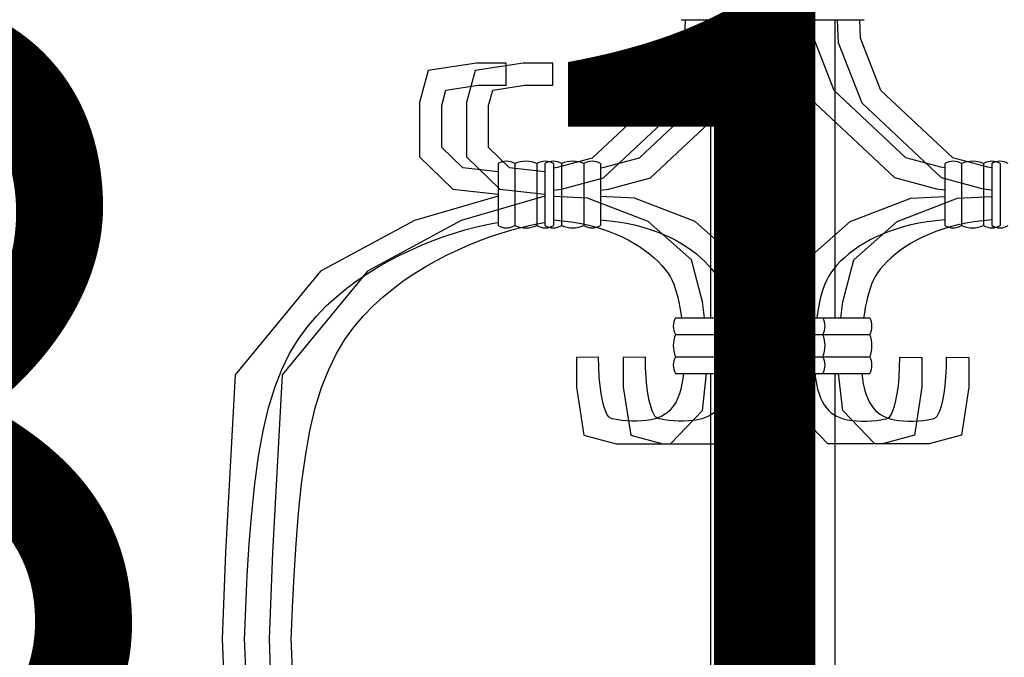
# Model space of a CAD drawing. Units: inches. Extents: x 2278 to 7495, y -71 to 1198.
# Tile 32 of 44: x 5127.04 to 5134.27, y 141.192 to 145.876. Entities that reach past the tile are written whole.
import ezdxf

# ---------------------------------------------------------------- set-up
doc = ezdxf.new("R2010")
doc.units = ezdxf.units.IN
doc.header["$MEASUREMENT"] = 0
doc.layers.add('A-ANNO-DIMS', color=2, linetype='Continuous', lineweight=18)
doc.layers.add('A-ELEV', color=7, linetype='Continuous', lineweight=25)
doc.styles.get("Standard").update_dxf_attribs({"font": 'arial.ttf'})
doc.dimstyles.get("Standard").update_dxf_attribs({"dimtxt": 6, "dimasz": 3, "dimexe": 0.18, "dimexo": 0.0625, "dimgap": 0.09, "dimtad": 0, "dimtih": 1, "dimtoh": 1, "dimdec": 0, "dimzin": 0, "dimdsep": 46, "dimlunit": 3, "dimtxsty": 'Standard', "dimblk": 'ARCHTICK', "dimcen": 0.09, "dimadec": 0, "dimazin": 0, "dimtfac": 1, "dimtdec": 0, "dimtofl": 0, "dimtmove": 0, "dimatfit": 3, "dimfxl": 1, "dimtolj": 1, "dimtzin": 0, "dimarcsym": 0})

# ---------------------------------------------------------------- blocks, each defined once
blk = doc.blocks.new('_ArchTick')
at = {"color": 0, "linetype": 'ByBlock', "const_width": 0.15}
blk.add_lwpolyline([(-0.5, -0.5), (0.5, 0.5)], dxfattribs=at)
blk = doc.blocks.new('*D59')
at = {"layer": 'A-ANNO-DIMS', "color": 0, "lineweight": -2, "transparency": 16777216}
for p, q in [((5096.5894, 159.1826), (5101.5644, 159.1826)), ((5101.3844, 159.1826), (5101.3844, 146.185)), ((5101.3844, 126.7988), (5101.3844, 139.7963)), ((5096.5894, 126.7988), (5101.5644, 126.7988))]:
    blk.add_line(p, q, dxfattribs=at)
at = {"layer": 'Defpoints', "color": 0, "transparency": 16777216}
for p in [(5096.5269, 159.1826), (5101.3844, 159.1826), (5096.5269, 126.7988)]:
    blk.add_point(p, dxfattribs=at)
at = {"layer": 'A-ANNO-DIMS', "color": 0, "lineweight": -2, "transparency": 16777216, "xscale": 3, "yscale": 3, "zscale": 3}
for p, rotation in [((5101.3844, 159.1826), 90), ((5101.3844, 126.7988), 270)]:
    blk.add_blockref('_ArchTick', p, dxfattribs=dict(at, rotation=rotation))
at = {"layer": 'A-ANNO-DIMS', "color": 0, "transparency": 16777216, "insert": (5101.3844, 142.9907), "char_height": 6, "attachment_point": 5}
blk.add_mtext('\\A1;ORNATE BALUSTER 2\'-8 1/2" TYP.', dxfattribs=at)
blk = doc.blocks.new('*D123')
at = {"layer": 'A-ANNO-DIMS', "color": 0, "lineweight": -2, "transparency": 16777216}
for p, q in [((4736.95, 340.1567), (4736.95, -23.4272)), ((5145.6762, -1.8097), (5145.6762, -23.4272)), ((4736.95, -23.2472), (4923.9291, -23.2472)), ((5145.6762, -23.2472), (4958.6971, -23.2472))]:
    blk.add_line(p, q, dxfattribs=at)
at = {"layer": 'Defpoints', "color": 0, "transparency": 16777216}
for p in [(4736.95, 340.2192), (5145.6762, -1.7472), (5145.6762, -23.2472)]:
    blk.add_point(p, dxfattribs=at)
at = {"layer": 'A-ANNO-DIMS', "color": 0, "lineweight": -2, "transparency": 16777216, "xscale": 3, "yscale": 3, "zscale": 3, "rotation": 180}
blk.add_blockref('_ArchTick', (4736.95, -23.2472), dxfattribs=at)
at = {"layer": 'A-ANNO-DIMS', "color": 0, "lineweight": -2, "transparency": 16777216, "xscale": 3, "yscale": 3, "zscale": 3}
blk.add_blockref('_ArchTick', (5145.6762, -23.2472), dxfattribs=at)
at = {"layer": 'A-ANNO-DIMS', "color": 0, "transparency": 16777216, "insert": (4941.3131, -23.2472), "char_height": 6, "attachment_point": 5}
blk.add_mtext('\\A1;34\'-0 1/2"', dxfattribs=at)
blk = doc.blocks.new('*D131')
at = {"layer": 'A-ANNO-DIMS', "color": 0, "lineweight": -2, "transparency": 16777216}
for p, q in [((5096.1762, 99.3153), (5096.1762, 361.8992)), ((5145.6762, 118.3153), (5145.6762, 361.8992)), ((5096.1762, 361.7192), (5105.7503, 361.7192)), ((5145.6762, 361.7192), (5136.1022, 361.7192))]:
    blk.add_line(p, q, dxfattribs=at)
at = {"layer": 'Defpoints', "color": 0, "transparency": 16777216}
for p in [(5145.6762, 361.7192), (5145.6762, 118.2528), (5096.1762, 99.2528)]:
    blk.add_point(p, dxfattribs=at)
at = {"layer": 'A-ANNO-DIMS', "color": 0, "lineweight": -2, "transparency": 16777216, "xscale": 3, "yscale": 3, "zscale": 3, "rotation": 180}
blk.add_blockref('_ArchTick', (5096.1762, 361.7192), dxfattribs=at)
at = {"layer": 'A-ANNO-DIMS', "color": 0, "lineweight": -2, "transparency": 16777216, "xscale": 3, "yscale": 3, "zscale": 3}
blk.add_blockref('_ArchTick', (5145.6762, 361.7192), dxfattribs=at)
at = {"layer": 'A-ANNO-DIMS', "color": 0, "transparency": 16777216, "insert": (5120.9262, 361.7192), "char_height": 6, "attachment_point": 5}
blk.add_mtext('\\A1;4\'-1 1/2"', dxfattribs=at)
blk = doc.blocks.new('*D139')
at = {"layer": 'A-ANNO-DIMS', "color": 0, "lineweight": -2, "transparency": 16777216}
for p, q in [((5092.2387, 160.2528), (5167.7538, 160.2528)), ((5167.5738, 160.2528), (5167.5738, 142.4083)), ((5167.5738, 118.2528), (5167.5738, 136.0973)), ((5145.7387, 118.2528), (5167.7538, 118.2528))]:
    blk.add_line(p, q, dxfattribs=at)
at = {"layer": 'Defpoints', "color": 0, "transparency": 16777216}
for p in [(5092.1762, 160.2528), (5167.5738, 160.2528), (5145.6762, 118.2528)]:
    blk.add_point(p, dxfattribs=at)
at = {"layer": 'A-ANNO-DIMS', "color": 0, "lineweight": -2, "transparency": 16777216, "xscale": 3, "yscale": 3, "zscale": 3}
for p, rotation in [((5167.5738, 160.2528), 90), ((5167.5738, 118.2528), 270)]:
    blk.add_blockref('_ArchTick', p, dxfattribs=dict(at, rotation=rotation))
at = {"layer": 'A-ANNO-DIMS', "color": 0, "transparency": 16777216, "insert": (5167.5738, 139.2528), "char_height": 6, "attachment_point": 5}
blk.add_mtext('\\A1;3\'-6"', dxfattribs=at)

msp = doc.modelspace()

# ---------------------------------------------------------------- linework, layer by layer
at = {"layer": 'A-ELEV'}
for p, q in [((5131.8965, 145.8765), (5132.8966, 145.8765)), ((5131.9226, 145.7411), (5131.9286, 145.8765)), ((5132.0842, 145.7072), (5132.0917, 145.8765)), ((5132.1114, 145.8765), (5132.1114, 143.6856)), ((5132.2404, 145.8765), (5133.2405, 145.8765)), ((5132.2665, 145.7411), (5132.2725, 145.8765)), ((5132.4281, 145.7072), (5132.4356, 145.8765)), ((5132.4553, 145.8765), (5132.4553, 143.6856)), ((5132.6817, 145.8765), (5132.6817, 143.6856)), ((5132.7089, 145.7072), (5132.7015, 145.8765)), ((5132.8705, 145.7411), (5132.8646, 145.8765)), ((5133.0256, 145.8765), (5133.0256, 143.6856)), ((5133.0528, 145.7072), (5133.0454, 145.8765)), ((5133.2144, 145.7411), (5133.2085, 145.8765)), ((5131.7733, 145.3557), (5131.9226, 145.7411)), ((5131.9118, 145.2623), (5132.0842, 145.7072)), ((5132.1172, 145.3557), (5132.2665, 145.7411)), ((5132.2557, 145.2623), (5132.4281, 145.7072)), ((5132.8813, 145.2623), (5132.7089, 145.7072)), ((5133.0199, 145.3557), (5132.8705, 145.7411)), ((5133.2252, 145.2623), (5133.0528, 145.7072)), ((5133.3638, 145.3557), (5133.2144, 145.7411)), ((5130.393, 145.5581), (5130.0391, 145.5036)), ((5130.7369, 145.5581), (5130.383, 145.5036)), ((5130.6107, 145.5581), (5130.393, 145.5581)), ((5130.6107, 145.3952), (5130.6107, 145.5581)), ((5130.9546, 145.5581), (5130.7369, 145.5581)), ((5130.9546, 145.3952), (5130.9546, 145.5581)), ((5130.0391, 145.5036), (5129.9756, 145.2675)), ((5130.383, 145.5036), (5130.3195, 145.2675)), ((5130.1386, 145.246), (5130.1689, 145.3587)), ((5130.1689, 145.3587), (5130.4054, 145.3952)), ((5130.4054, 145.3952), (5130.6107, 145.3952)), ((5130.4825, 145.246), (5130.5128, 145.3587)), ((5130.5128, 145.3587), (5130.7493, 145.3952)), ((5130.7493, 145.3952), (5130.9546, 145.3952)), ((5131.2459, 144.8607), (5131.7733, 145.3557)), ((5131.5898, 144.8607), (5132.1172, 145.3557)), ((5133.5472, 144.8607), (5133.0199, 145.3557)), ((5133.8911, 144.8607), (5133.3638, 145.3557)), ((5129.9756, 145.2675), (5129.9756, 144.868)), ((5130.3195, 145.2675), (5130.3195, 144.868)), ((5131.3274, 144.7137), (5131.9118, 145.2623)), ((5131.6713, 144.7137), (5132.2557, 145.2623)), ((5133.4657, 144.7137), (5132.8813, 145.2623)), ((5133.8096, 144.7137), (5133.2252, 145.2623)), ((5130.1386, 144.9373), (5130.1386, 145.246)), ((5130.4825, 144.9373), (5130.4825, 145.246)), ((5130.2936, 144.7879), (5130.1386, 144.9373)), ((5130.6375, 144.7879), (5130.4825, 144.9373)), ((5129.9756, 144.868), (5130.2206, 144.632)), ((5130.3195, 144.868), (5130.5645, 144.632)), ((5130.5528, 144.8198), (5130.5528, 144.3639)), ((5130.675, 144.8198), (5130.675, 144.3639)), ((5130.838, 144.8198), (5130.838, 144.3639)), ((5130.8967, 144.8198), (5130.8967, 144.3639)), ((5130.9602, 144.8198), (5130.9602, 144.3639)), ((5130.9883, 144.7924), (5131.2459, 144.8607)), ((5131.0189, 144.8198), (5131.0189, 144.3639)), ((5131.1819, 144.8198), (5131.1819, 144.3639)), ((5131.3041, 144.8198), (5131.3041, 144.3639)), ((5131.3322, 144.7924), (5131.5898, 144.8607)), ((5133.8048, 144.7924), (5133.5472, 144.8607)), ((5133.833, 144.8198), (5133.833, 144.3639)), ((5134.1487, 144.7924), (5133.8911, 144.8607)), ((5133.9552, 144.8198), (5133.9552, 144.3639)), ((5134.1181, 144.8198), (5134.1181, 144.3639)), ((5134.1769, 144.8198), (5134.1769, 144.3639)), ((5134.2403, 144.8198), (5134.2403, 144.3639)), ((5130.5528, 144.7597), (5130.2936, 144.7879)), ((5130.8967, 144.7597), (5130.6375, 144.7879)), ((5130.9602, 144.7891), (5130.9883, 144.7924)), ((5131.3041, 144.7891), (5131.3322, 144.7924)), ((5133.833, 144.7891), (5133.8048, 144.7924)), ((5134.1769, 144.7891), (5134.1487, 144.7924)), ((5131.019, 144.632), (5131.3274, 144.7137)), ((5131.3629, 144.632), (5131.6713, 144.7137)), ((5133.7742, 144.632), (5133.4657, 144.7137)), ((5134.1181, 144.632), (5133.8096, 144.7137)), ((5130.2206, 144.632), (5130.5528, 144.5958)), ((5130.5645, 144.632), (5130.8967, 144.5958)), ((5130.9602, 144.625), (5131.019, 144.632)), ((5131.3041, 144.625), (5131.3629, 144.632)), ((5133.833, 144.625), (5133.7742, 144.632)), ((5134.1769, 144.625), (5134.1181, 144.632)), ((5130.5528, 144.581), (5129.9387, 144.402)), ((5130.8967, 144.581), (5130.2826, 144.402)), ((5131.2098, 144.5653), (5130.9602, 144.5763)), ((5131.6547, 144.3929), (5131.2098, 144.5653)), ((5131.5537, 144.5653), (5131.3041, 144.5763)), ((5131.9986, 144.3929), (5131.5537, 144.5653)), ((5133.1384, 144.3929), (5133.5833, 144.5653)), ((5133.4823, 144.3929), (5133.9272, 144.5653)), ((5133.5833, 144.5653), (5133.833, 144.5763)), ((5133.9272, 144.5653), (5134.1769, 144.5763)), ((5129.9387, 144.402), (5129.2486, 144.03)), ((5130.2826, 144.402), (5129.5925, 144.03)), ((5130.5338, 144.3836), (5130.5528, 144.3865)), ((5130.8777, 144.3836), (5130.8967, 144.3865)), ((5130.9602, 144.405), (5131.0258, 144.3993)), ((5131.0258, 144.3993), (5131.0896, 144.3912)), ((5131.0896, 144.3912), (5131.1509, 144.3809)), ((5131.3041, 144.405), (5131.3697, 144.3993)), ((5131.3697, 144.3993), (5131.4335, 144.3912)), ((5131.4335, 144.3912), (5131.4948, 144.3809)), ((5131.9725, 144.1117), (5131.6547, 144.3929)), ((5132.3164, 144.1117), (5131.9986, 144.3929)), ((5132.8207, 144.1117), (5133.1384, 144.3929)), ((5133.1646, 144.1117), (5133.4823, 144.3929)), ((5133.7035, 144.3912), (5133.6422, 144.3809)), ((5133.7673, 144.3993), (5133.7035, 144.3912)), ((5133.833, 144.405), (5133.7673, 144.3993)), ((5134.0474, 144.3912), (5133.9861, 144.3809)), ((5134.1112, 144.3993), (5134.0474, 144.3912)), ((5134.1769, 144.405), (5134.1112, 144.3993)), ((5130.2316, 144.3089), (5130.3086, 144.3322)), ((5130.3086, 144.3322), (5130.3846, 144.3524)), ((5130.3846, 144.3524), (5130.4597, 144.3696)), ((5130.4597, 144.3696), (5130.5338, 144.3836)), ((5130.5755, 144.3089), (5130.6525, 144.3322)), ((5130.6525, 144.3322), (5130.7285, 144.3524)), ((5130.7285, 144.3524), (5130.8036, 144.3696)), ((5130.8036, 144.3696), (5130.8777, 144.3836)), ((5131.1509, 144.3809), (5131.2094, 144.3687)), ((5131.2094, 144.3687), (5131.2652, 144.3546)), ((5131.2652, 144.3546), (5131.3184, 144.3387)), ((5131.3184, 144.3387), (5131.3691, 144.3211)), ((5131.3691, 144.3211), (5131.4175, 144.3018)), ((5131.4948, 144.3809), (5131.5534, 144.3687)), ((5131.5534, 144.3687), (5131.6091, 144.3546)), ((5131.6091, 144.3546), (5131.6623, 144.3387)), ((5131.6623, 144.3387), (5131.713, 144.3211)), ((5131.713, 144.3211), (5131.7614, 144.3018)), ((5133.424, 144.3211), (5133.3756, 144.3018)), ((5133.4747, 144.3387), (5133.424, 144.3211)), ((5133.5279, 144.3546), (5133.4747, 144.3387)), ((5133.5837, 144.3687), (5133.5279, 144.3546)), ((5133.6422, 144.3809), (5133.5837, 144.3687)), ((5133.7679, 144.3211), (5133.7195, 144.3018)), ((5133.8186, 144.3387), (5133.7679, 144.3211)), ((5133.8718, 144.3546), (5133.8186, 144.3387)), ((5133.9276, 144.3687), (5133.8718, 144.3546)), ((5133.9861, 144.3809), (5133.9276, 144.3687)), ((5129.9956, 144.2214), (5130.0751, 144.2535)), ((5130.0751, 144.2535), (5130.1538, 144.2827)), ((5130.1538, 144.2827), (5130.2316, 144.3089)), ((5130.3395, 144.2214), (5130.419, 144.2535)), ((5130.419, 144.2535), (5130.4977, 144.2827)), ((5130.4977, 144.2827), (5130.5755, 144.3089)), ((5131.4175, 144.3018), (5131.4637, 144.281)), ((5131.4637, 144.281), (5131.5079, 144.2586)), ((5131.5079, 144.2586), (5131.5502, 144.2347)), ((5131.7614, 144.3018), (5131.8076, 144.281)), ((5131.8076, 144.281), (5131.8518, 144.2586)), ((5131.8518, 144.2586), (5131.8941, 144.2347)), ((5133.2852, 144.2586), (5133.2429, 144.2347)), ((5133.3294, 144.281), (5133.2852, 144.2586)), ((5133.3756, 144.3018), (5133.3294, 144.281)), ((5133.6291, 144.2586), (5133.5868, 144.2347)), ((5133.6733, 144.281), (5133.6291, 144.2586)), ((5133.7195, 144.3018), (5133.6733, 144.281)), ((5129.8357, 144.149), (5129.9156, 144.1867)), ((5129.9156, 144.1867), (5129.9956, 144.2214)), ((5130.1796, 144.149), (5130.2595, 144.1867)), ((5130.2595, 144.1867), (5130.3395, 144.2214)), ((5131.5502, 144.2347), (5131.5906, 144.2094)), ((5131.5906, 144.2094), (5131.6288, 144.183)), ((5131.6288, 144.183), (5131.6645, 144.1557)), ((5131.8941, 144.2347), (5131.9345, 144.2094)), ((5131.9345, 144.2094), (5131.9727, 144.183)), ((5131.9727, 144.183), (5132.0084, 144.1557)), ((5133.1644, 144.183), (5133.1286, 144.1557)), ((5133.2026, 144.2094), (5133.1644, 144.183)), ((5133.2429, 144.2347), (5133.2026, 144.2094)), ((5133.5083, 144.183), (5133.4725, 144.1557)), ((5133.5465, 144.2094), (5133.5083, 144.183)), ((5133.5868, 144.2347), (5133.5465, 144.2094)), ((5129.6768, 144.0636), (5129.7561, 144.1081)), ((5129.7561, 144.1081), (5129.8357, 144.149)), ((5130.0207, 144.0636), (5130.1, 144.1081)), ((5130.1, 144.1081), (5130.1796, 144.149)), ((5131.6645, 144.1557), (5131.6975, 144.1278)), ((5131.6975, 144.1278), (5131.7276, 144.0995)), ((5131.7276, 144.0995), (5131.7545, 144.0712)), ((5132.0542, 143.8032), (5131.9725, 144.1117)), ((5132.0084, 144.1557), (5132.0414, 144.1278)), ((5132.0414, 144.1278), (5132.0715, 144.0995)), ((5132.0715, 144.0995), (5132.0984, 144.0712)), ((5132.3981, 143.8032), (5132.3164, 144.1117)), ((5132.7389, 143.8032), (5132.8207, 144.1117)), ((5133.0655, 144.0995), (5133.0386, 144.0712)), ((5133.0956, 144.1278), (5133.0655, 144.0995)), ((5133.0828, 143.8032), (5133.1646, 144.1117)), ((5133.1286, 144.1557), (5133.0956, 144.1278)), ((5133.4094, 144.0995), (5133.3825, 144.0712)), ((5133.4395, 144.1278), (5133.4094, 144.0995)), ((5133.4725, 144.1557), (5133.4395, 144.1278)), ((5129.2486, 144.03), (5128.6221, 143.2679)), ((5129.5925, 144.03), (5128.966, 143.2679)), ((5129.598, 144.0151), (5129.6768, 144.0636)), ((5129.942, 144.0151), (5130.0207, 144.0636)), ((5131.7545, 144.0712), (5131.7781, 144.0431)), ((5131.7781, 144.0431), (5131.7981, 144.0157)), ((5132.0984, 144.0712), (5132.122, 144.0431)), ((5132.122, 144.0431), (5132.142, 144.0157)), ((5133.0151, 144.0431), (5132.995, 144.0157)), ((5133.0386, 144.0712), (5133.0151, 144.0431)), ((5133.359, 144.0431), (5133.3389, 144.0157)), ((5133.3825, 144.0712), (5133.359, 144.0431)), ((5129.4423, 143.9045), (5129.5199, 143.9622)), ((5129.5199, 143.9622), (5129.598, 144.0151)), ((5129.7862, 143.9045), (5129.8638, 143.9622)), ((5129.8638, 143.9622), (5129.942, 144.0151)), ((5131.7981, 144.0157), (5131.815, 143.9886)), ((5131.815, 143.9886), (5131.8296, 143.9612)), ((5131.8296, 143.9612), (5131.8422, 143.9327)), ((5132.142, 144.0157), (5132.159, 143.9886)), ((5132.159, 143.9886), (5132.1735, 143.9612)), ((5132.1735, 143.9612), (5132.1861, 143.9327)), ((5132.9635, 143.9612), (5132.9509, 143.9327)), ((5132.9781, 143.9886), (5132.9635, 143.9612)), ((5132.995, 144.0157), (5132.9781, 143.9886)), ((5133.3074, 143.9612), (5133.2948, 143.9327)), ((5133.322, 143.9886), (5133.3074, 143.9612)), ((5133.3389, 144.0157), (5133.322, 143.9886)), ((5129.3657, 143.8416), (5129.4423, 143.9045)), ((5129.7096, 143.8416), (5129.7862, 143.9045)), ((5131.8422, 143.9327), (5131.8534, 143.9027)), ((5131.8534, 143.9027), (5131.8633, 143.8709)), ((5132.1861, 143.9327), (5132.1973, 143.9027)), ((5132.1973, 143.9027), (5132.2072, 143.8709)), ((5132.9397, 143.9027), (5132.9298, 143.8709)), ((5132.9509, 143.9327), (5132.9397, 143.9027)), ((5133.2836, 143.9027), (5133.2737, 143.8709)), ((5133.2948, 143.9327), (5133.2836, 143.9027)), ((5129.2908, 143.7735), (5129.3657, 143.8416)), ((5129.6347, 143.7735), (5129.7096, 143.8416)), ((5131.8633, 143.8709), (5131.8722, 143.8368)), ((5131.8722, 143.8368), (5131.8803, 143.8003)), ((5132.2072, 143.8709), (5132.2161, 143.8368)), ((5132.2161, 143.8368), (5132.2242, 143.8003)), ((5132.9209, 143.8368), (5132.9128, 143.8003)), ((5132.9298, 143.8709), (5132.9209, 143.8368)), ((5133.2648, 143.8368), (5133.2567, 143.8003)), ((5133.2737, 143.8709), (5133.2648, 143.8368)), ((5129.2186, 143.6994), (5129.2908, 143.7735)), ((5129.5625, 143.6994), (5129.6347, 143.7735)), ((5131.8803, 143.8003), (5131.8879, 143.7615)), ((5131.8879, 143.7615), (5131.895, 143.7208)), ((5132.0682, 143.6856), (5132.0542, 143.8032)), ((5132.2242, 143.8003), (5132.2318, 143.7615)), ((5132.2318, 143.7615), (5132.2389, 143.7208)), ((5132.4121, 143.6856), (5132.3981, 143.8032)), ((5132.7249, 143.6856), (5132.7389, 143.8032)), ((5132.9052, 143.7615), (5132.8981, 143.7208)), ((5132.9128, 143.8003), (5132.9052, 143.7615)), ((5133.0688, 143.6856), (5133.0828, 143.8032)), ((5133.2491, 143.7615), (5133.242, 143.7208)), ((5133.2567, 143.8003), (5133.2491, 143.7615)), ((5129.1494, 143.6175), (5129.2186, 143.6994)), ((5129.4933, 143.6175), (5129.5625, 143.6994)), ((5131.8558, 143.6856), (5132.9373, 143.6856)), ((5131.895, 143.7208), (5131.9005, 143.6856)), ((5132.1997, 143.6856), (5133.2812, 143.6856)), ((5132.2389, 143.7208), (5132.2444, 143.6856)), ((5132.8981, 143.7208), (5132.8926, 143.6856)), ((5133.242, 143.7208), (5133.2365, 143.6856)), ((5129.0837, 143.5262), (5129.1494, 143.6175)), ((5129.4276, 143.5262), (5129.4933, 143.6175)), ((5129.0219, 143.4234), (5129.0837, 143.5262)), ((5129.3658, 143.4234), (5129.4276, 143.5262)), ((5131.8558, 143.5634), (5132.9373, 143.5634)), ((5132.1997, 143.5634), (5133.2812, 143.5634)), ((5128.9646, 143.3071), (5129.0219, 143.4234)), ((5129.3085, 143.3071), (5129.3658, 143.4234)), ((5131.291, 143.3975), (5131.1281, 143.3949)), ((5131.1281, 143.3949), (5131.1281, 143.1772)), ((5131.2922, 143.3207), (5131.291, 143.3975)), ((5131.6349, 143.3975), (5131.472, 143.3949)), ((5131.472, 143.3949), (5131.472, 143.1772)), ((5131.6361, 143.3207), (5131.6349, 143.3975)), ((5131.8558, 143.4004), (5132.9373, 143.4004)), ((5132.1997, 143.4004), (5133.2812, 143.4004)), ((5133.5009, 143.3207), (5133.5021, 143.3975)), ((5133.5021, 143.3975), (5133.6651, 143.3949)), ((5133.6651, 143.3949), (5133.6651, 143.1772)), ((5133.8448, 143.3207), (5133.846, 143.3975)), ((5133.846, 143.3975), (5134.009, 143.3949)), ((5134.009, 143.3949), (5134.009, 143.1772)), ((5128.9124, 143.1752), (5128.9646, 143.3071)), ((5129.2563, 143.1752), (5129.3085, 143.3071)), ((5131.2957, 143.2512), (5131.2922, 143.3207)), ((5131.6396, 143.2512), (5131.6361, 143.3207)), ((5133.4974, 143.2512), (5133.5009, 143.3207)), ((5133.8413, 143.2512), (5133.8448, 143.3207)), ((5128.6221, 143.2679), (5128.5514, 141.9615)), ((5128.966, 143.2679), (5128.8953, 141.9615)), ((5131.3015, 143.1873), (5131.2957, 143.2512)), ((5131.6454, 143.1873), (5131.6396, 143.2512)), ((5131.8558, 143.2782), (5132.9373, 143.2782)), ((5131.9098, 143.2403), (5131.9029, 143.2002)), ((5131.9146, 143.2782), (5131.9098, 143.2403)), ((5132.0542, 143.0048), (5132.0839, 143.2782)), ((5132.1114, 143.2782), (5132.1114, 139.3773)), ((5132.1997, 143.2782), (5133.2812, 143.2782)), ((5132.2537, 143.2403), (5132.2468, 143.2002)), ((5132.2585, 143.2782), (5132.2537, 143.2403)), ((5132.3981, 143.0048), (5132.4278, 143.2782)), ((5132.4553, 143.2782), (5132.4553, 139.3773)), ((5132.6817, 143.2782), (5132.6817, 139.3773)), ((5132.7389, 143.0048), (5132.7092, 143.2782)), ((5132.8786, 143.2782), (5132.8833, 143.2403)), ((5132.8833, 143.2403), (5132.8903, 143.2002)), ((5133.0256, 143.2782), (5133.0256, 139.3773)), ((5133.0828, 143.0048), (5133.0531, 143.2782)), ((5133.2225, 143.2782), (5133.2272, 143.2403)), ((5133.2272, 143.2403), (5133.2342, 143.2002)), ((5133.4917, 143.1873), (5133.4974, 143.2512)), ((5133.8356, 143.1873), (5133.8413, 143.2512)), ((5128.8662, 143.0257), (5128.9124, 143.1752)), ((5129.2101, 143.0257), (5129.2563, 143.1752)), ((5131.1281, 143.1772), (5131.1826, 142.8234)), ((5131.3092, 143.1295), (5131.3015, 143.1873)), ((5131.472, 143.1772), (5131.5265, 142.8234)), ((5131.6531, 143.1295), (5131.6454, 143.1873)), ((5131.8942, 143.1627), (5131.884, 143.1283)), ((5131.9029, 143.2002), (5131.8942, 143.1627)), ((5132.2381, 143.1627), (5132.2279, 143.1283)), ((5132.2468, 143.2002), (5132.2381, 143.1627)), ((5132.8903, 143.2002), (5132.8989, 143.1627)), ((5132.8989, 143.1627), (5132.9091, 143.1283)), ((5133.2342, 143.2002), (5133.2428, 143.1627)), ((5133.2428, 143.1627), (5133.253, 143.1283)), ((5133.4839, 143.1295), (5133.4917, 143.1873)), ((5133.6651, 143.1772), (5133.6106, 142.8234)), ((5133.8278, 143.1295), (5133.8356, 143.1873)), ((5134.009, 143.1772), (5133.9545, 142.8234)), ((5131.3188, 143.0788), (5131.3092, 143.1295)), ((5131.6627, 143.0788), (5131.6531, 143.1295)), ((5131.8724, 143.0975), (5131.8594, 143.0702)), ((5131.884, 143.1283), (5131.8724, 143.0975)), ((5132.2163, 143.0975), (5132.2033, 143.0702)), ((5132.2279, 143.1283), (5132.2163, 143.0975)), ((5132.9091, 143.1283), (5132.9207, 143.0975)), ((5132.9207, 143.0975), (5132.9337, 143.0702)), ((5133.253, 143.1283), (5133.2646, 143.0975)), ((5133.2646, 143.0975), (5133.2776, 143.0702)), ((5133.4743, 143.0788), (5133.4839, 143.1295)), ((5133.8182, 143.0788), (5133.8278, 143.1295)), ((5128.8267, 142.8565), (5128.8662, 143.0257)), ((5129.1706, 142.8565), (5129.2101, 143.0257)), ((5131.3297, 143.036), (5131.3188, 143.0788)), ((5131.3412, 143.0023), (5131.3297, 143.036)), ((5131.6736, 143.036), (5131.6627, 143.0788)), ((5131.6851, 143.0023), (5131.6736, 143.036)), ((5131.8294, 143.0245), (5131.8127, 143.0057)), ((5131.845, 143.0459), (5131.8294, 143.0245)), ((5131.8594, 143.0702), (5131.845, 143.0459)), ((5132.1733, 143.0245), (5132.1566, 143.0057)), ((5132.1889, 143.0459), (5132.1733, 143.0245)), ((5132.2033, 143.0702), (5132.1889, 143.0459)), ((5132.9337, 143.0702), (5132.9481, 143.0459)), ((5132.9481, 143.0459), (5132.9637, 143.0245)), ((5132.9637, 143.0245), (5132.9805, 143.0057)), ((5133.2776, 143.0702), (5133.292, 143.0459)), ((5133.292, 143.0459), (5133.3076, 143.0245)), ((5133.3076, 143.0245), (5133.3244, 143.0057)), ((5133.4519, 143.0023), (5133.4634, 143.036)), ((5133.4634, 143.036), (5133.4743, 143.0788)), ((5133.7958, 143.0023), (5133.8073, 143.036)), ((5133.8073, 143.036), (5133.8182, 143.0788)), ((5131.352, 142.9788), (5131.3412, 143.0023)), ((5131.3607, 142.9648), (5131.352, 142.9788)), ((5131.367, 142.9576), (5131.3607, 142.9648)), ((5131.3721, 142.9534), (5131.367, 142.9576)), ((5131.3786, 142.9496), (5131.3721, 142.9534)), ((5131.3895, 142.9453), (5131.3786, 142.9496)), ((5131.4069, 142.9406), (5131.3895, 142.9453)), ((5131.4313, 142.9363), (5131.4069, 142.9406)), ((5131.7059, 142.9443), (5131.6761, 142.9373)), ((5131.6959, 142.9788), (5131.6851, 143.0023)), ((5131.7046, 142.9648), (5131.6959, 142.9788)), ((5131.7109, 142.9576), (5131.7046, 142.9648)), ((5131.732, 142.9528), (5131.7059, 142.9443)), ((5131.716, 142.9534), (5131.7109, 142.9576)), ((5131.7225, 142.9496), (5131.716, 142.9534)), ((5131.7334, 142.9453), (5131.7225, 142.9496)), ((5131.7548, 142.963), (5131.732, 142.9528)), ((5131.7508, 142.9406), (5131.7334, 142.9453)), ((5131.7753, 142.9363), (5131.7508, 142.9406)), ((5131.7756, 142.9751), (5131.7548, 142.963)), ((5131.7948, 142.9893), (5131.7756, 142.9751)), ((5131.8127, 143.0057), (5131.7948, 142.9893)), ((5131.8181, 142.7599), (5132.0542, 143.0048)), ((5132.0498, 142.9443), (5132.02, 142.9373)), ((5132.0759, 142.9528), (5132.0498, 142.9443)), ((5132.0987, 142.963), (5132.0759, 142.9528)), ((5132.1195, 142.9751), (5132.0987, 142.963)), ((5132.1387, 142.9893), (5132.1195, 142.9751)), ((5132.1566, 143.0057), (5132.1387, 142.9893)), ((5132.162, 142.7599), (5132.3981, 143.0048)), ((5132.975, 142.7599), (5132.7389, 143.0048)), ((5132.9805, 143.0057), (5132.9984, 142.9893)), ((5132.9984, 142.9893), (5133.0176, 142.9751)), ((5133.0176, 142.9751), (5133.0383, 142.963)), ((5133.0383, 142.963), (5133.0611, 142.9528)), ((5133.0611, 142.9528), (5133.0872, 142.9443)), ((5133.3189, 142.7599), (5133.0828, 143.0048)), ((5133.0872, 142.9443), (5133.117, 142.9373)), ((5133.3244, 143.0057), (5133.3423, 142.9893)), ((5133.3423, 142.9893), (5133.3615, 142.9751)), ((5133.3615, 142.9751), (5133.3822, 142.963)), ((5133.3618, 142.9363), (5133.3862, 142.9406)), ((5133.3822, 142.963), (5133.405, 142.9528)), ((5133.3862, 142.9406), (5133.4036, 142.9453)), ((5133.4036, 142.9453), (5133.4146, 142.9496)), ((5133.405, 142.9528), (5133.4311, 142.9443)), ((5133.4146, 142.9496), (5133.4211, 142.9534)), ((5133.4211, 142.9534), (5133.4261, 142.9576)), ((5133.4261, 142.9576), (5133.4324, 142.9648)), ((5133.4311, 142.9443), (5133.4609, 142.9373)), ((5133.4324, 142.9648), (5133.4411, 142.9788)), ((5133.4411, 142.9788), (5133.4519, 143.0023)), ((5133.7057, 142.9363), (5133.7301, 142.9406)), ((5133.7301, 142.9406), (5133.7475, 142.9453)), ((5133.7475, 142.9453), (5133.7585, 142.9496)), ((5133.7585, 142.9496), (5133.765, 142.9534)), ((5133.765, 142.9534), (5133.77, 142.9576)), ((5133.77, 142.9576), (5133.7763, 142.9648)), ((5133.7763, 142.9648), (5133.785, 142.9788)), ((5133.785, 142.9788), (5133.7958, 143.0023)), ((5131.4623, 142.9326), (5131.4313, 142.9363)), ((5131.4975, 142.9296), (5131.4623, 142.9326)), ((5131.5342, 142.9279), (5131.4975, 142.9296)), ((5131.5713, 142.9276), (5131.5342, 142.9279)), ((5131.6079, 142.9289), (5131.5713, 142.9276)), ((5131.6431, 142.9322), (5131.6079, 142.9289)), ((5131.6761, 142.9373), (5131.6431, 142.9322)), ((5131.8062, 142.9326), (5131.7753, 142.9363)), ((5131.8414, 142.9296), (5131.8062, 142.9326)), ((5131.8781, 142.9279), (5131.8414, 142.9296)), ((5131.9152, 142.9276), (5131.8781, 142.9279)), ((5131.9518, 142.9289), (5131.9152, 142.9276)), ((5131.987, 142.9322), (5131.9518, 142.9289)), ((5132.02, 142.9373), (5131.987, 142.9322)), ((5133.117, 142.9373), (5133.15, 142.9322)), ((5133.15, 142.9322), (5133.1853, 142.9289)), ((5133.1853, 142.9289), (5133.2219, 142.9276)), ((5133.2219, 142.9276), (5133.259, 142.9279)), ((5133.259, 142.9279), (5133.2957, 142.9296)), ((5133.2957, 142.9296), (5133.3308, 142.9326)), ((5133.3308, 142.9326), (5133.3618, 142.9363)), ((5133.4609, 142.9373), (5133.4939, 142.9322)), ((5133.4939, 142.9322), (5133.5292, 142.9289)), ((5133.5292, 142.9289), (5133.5658, 142.9276)), ((5133.5658, 142.9276), (5133.6029, 142.9279)), ((5133.6029, 142.9279), (5133.6396, 142.9296)), ((5133.6396, 142.9296), (5133.6747, 142.9326)), ((5133.6747, 142.9326), (5133.7057, 142.9363)), ((5128.7934, 142.6689), (5128.8267, 142.8565)), ((5129.1373, 142.6689), (5129.1706, 142.8565)), ((5131.1826, 142.8234), (5131.4186, 142.7599)), ((5131.5265, 142.8234), (5131.7625, 142.7599)), ((5133.6106, 142.8234), (5133.3745, 142.7599)), ((5133.9545, 142.8234), (5133.7184, 142.7599)), ((5131.4186, 142.7599), (5131.8181, 142.7599)), ((5131.7625, 142.7599), (5132.162, 142.7599)), ((5133.3745, 142.7599), (5132.975, 142.7599)), ((5133.7184, 142.7599), (5133.3189, 142.7599)), ((5128.7659, 142.466), (5128.7934, 142.6689)), ((5129.1098, 142.466), (5129.1373, 142.6689)), ((5128.7435, 142.2507), (5128.7659, 142.466)), ((5129.0874, 142.2507), (5129.1098, 142.466)), ((5128.7255, 142.0258), (5128.7435, 142.2507)), ((5129.0694, 142.0258), (5129.0874, 142.2507)), ((5128.7111, 141.7942), (5128.7255, 142.0258)), ((5129.055, 141.7942), (5129.0694, 142.0258)), ((5128.5514, 141.9615), (5128.5267, 141.3278)), ((5128.8953, 141.9615), (5128.8706, 141.3278)), ((5128.6994, 141.5585), (5128.7111, 141.7942)), ((5129.0433, 141.5585), (5129.055, 141.7942)), ((5128.6895, 141.321), (5128.6994, 141.5585)), ((5129.0334, 141.321), (5129.0433, 141.5585)), ((5128.5267, 141.3278), (5128.5514, 140.694)), ((5128.6994, 141.0971), (5128.6895, 141.3345)), ((5128.8706, 141.3278), (5128.8953, 140.694)), ((5129.0433, 141.0971), (5129.0334, 141.3345))]:
    msp.add_line(p, q, dxfattribs=at)
for centre, radius, start, end in [((5130.6139, 144.7149), 0.1214, 59.77678, 120.22322), ((5130.7565, 144.627), 0.2094, 67.10166, 112.89834), ((5130.8991, 144.7149), 0.1214, 59.77678, 120.22322), ((5130.9578, 144.7149), 0.1214, 59.77678, 120.22322), ((5131.1004, 144.627), 0.2094, 67.10166, 112.89834), ((5131.243, 144.7149), 0.1214, 59.77678, 120.22322), ((5133.8941, 144.7149), 0.1214, 59.77678, 120.22322), ((5134.0366, 144.627), 0.2094, 67.10166, 112.89834), ((5134.1792, 144.7149), 0.1214, 59.77678, 120.22322), ((5134.238, 144.7149), 0.1214, 59.77678, 120.22322), ((5130.6139, 144.4688), 0.1214, 239.77678, 300.22322), ((5130.7565, 144.5568), 0.2094, 247.10166, 292.89834), ((5130.8991, 144.4688), 0.1214, 239.77678, 300.22322), ((5130.9578, 144.4688), 0.1214, 239.77678, 300.22322), ((5131.1004, 144.5568), 0.2094, 247.10166, 292.89834), ((5131.243, 144.4688), 0.1214, 239.77678, 300.22322), ((5133.8941, 144.4688), 0.1214, 239.77678, 300.22322), ((5134.0366, 144.5568), 0.2094, 247.10166, 292.89834), ((5134.1792, 144.4688), 0.1214, 239.77678, 300.22322), ((5134.238, 144.4688), 0.1214, 239.77678, 300.22322), ((5131.9607, 143.6245), 0.1214, 149.77678, 210.22322), ((5132.3046, 143.6245), 0.1214, 149.77678, 210.22322), ((5132.8324, 143.6245), 0.1214, 329.77678, 30.22322), ((5133.1764, 143.6245), 0.1214, 329.77678, 30.22322), ((5132.0487, 143.4819), 0.2094, 157.10166, 202.89834), ((5132.3926, 143.4819), 0.2094, 157.10166, 202.89834), ((5132.7445, 143.4819), 0.2094, 337.10166, 22.89834), ((5133.0884, 143.4819), 0.2094, 337.10166, 22.89834), ((5131.9607, 143.3393), 0.1214, 149.77678, 210.22322), ((5132.3046, 143.3393), 0.1214, 149.77678, 210.22322), ((5132.8324, 143.3393), 0.1214, 329.77678, 30.22322), ((5133.1764, 143.3393), 0.1214, 329.77678, 30.22322)]:
    msp.add_arc(centre, radius, start, end, dxfattribs=at)

# ---------------------------------------------------------------- dimensions: what is measured, and where the dimension line sits
at = {"layer": 'A-ANNO-DIMS'}
for base, p1, p2, picture, middle in [((5145.6762, 361.7192), (5096.1762, 99.2528), (5145.6762, 118.2528), '*D131', (5120.9262, 361.7192)), ((5145.6762, -23.2472), (4736.95, 340.2192), (5145.6762, -1.7472), '*D123', (4941.3131, -23.2472))]:
    dim = msp.add_linear_dim(base=base, p1=p1, p2=p2, dimstyle='Standard', override={"dimdec": 1, "dimlfac": 1, "dimrnd": 0, "dimzin": 1, "dimdsep": 46, "dimlunit": 4, "dimfrac": 2}, dxfattribs=at)
    dim.commit()
    dim.dimension.update_dxf_attribs({"geometry": picture, "text_midpoint": middle})
dim = msp.add_linear_dim(base=(5101.3844, 159.1826), p1=(5096.5269, 126.7988), p2=(5096.5269, 159.1826), angle=90, text='ORNATE BALUSTER <> TYP.', dimstyle='Standard', override={"dimdec": 1, "dimrnd": 0, "dimzin": 1, "dimlunit": 4, "dimfrac": 2}, dxfattribs=at)
dim.commit()
dim.dimension.update_dxf_attribs({"geometry": '*D59', "text_midpoint": (5101.3844, 142.9907)})
dim = msp.add_linear_dim(base=(5167.5738, 160.2528), p1=(5145.6762, 118.2528), p2=(5092.1762, 160.2528), angle=90, dimstyle='Standard', override={"dimdec": 1, "dimlfac": 1, "dimrnd": 0, "dimzin": 1, "dimdsep": 46, "dimlunit": 4, "dimfrac": 2}, dxfattribs=at)
dim.commit()
dim.dimension.update_dxf_attribs({"geometry": '*D139', "text_midpoint": (5167.5738, 139.2528)})

doc.saveas('drawing.dxf')
